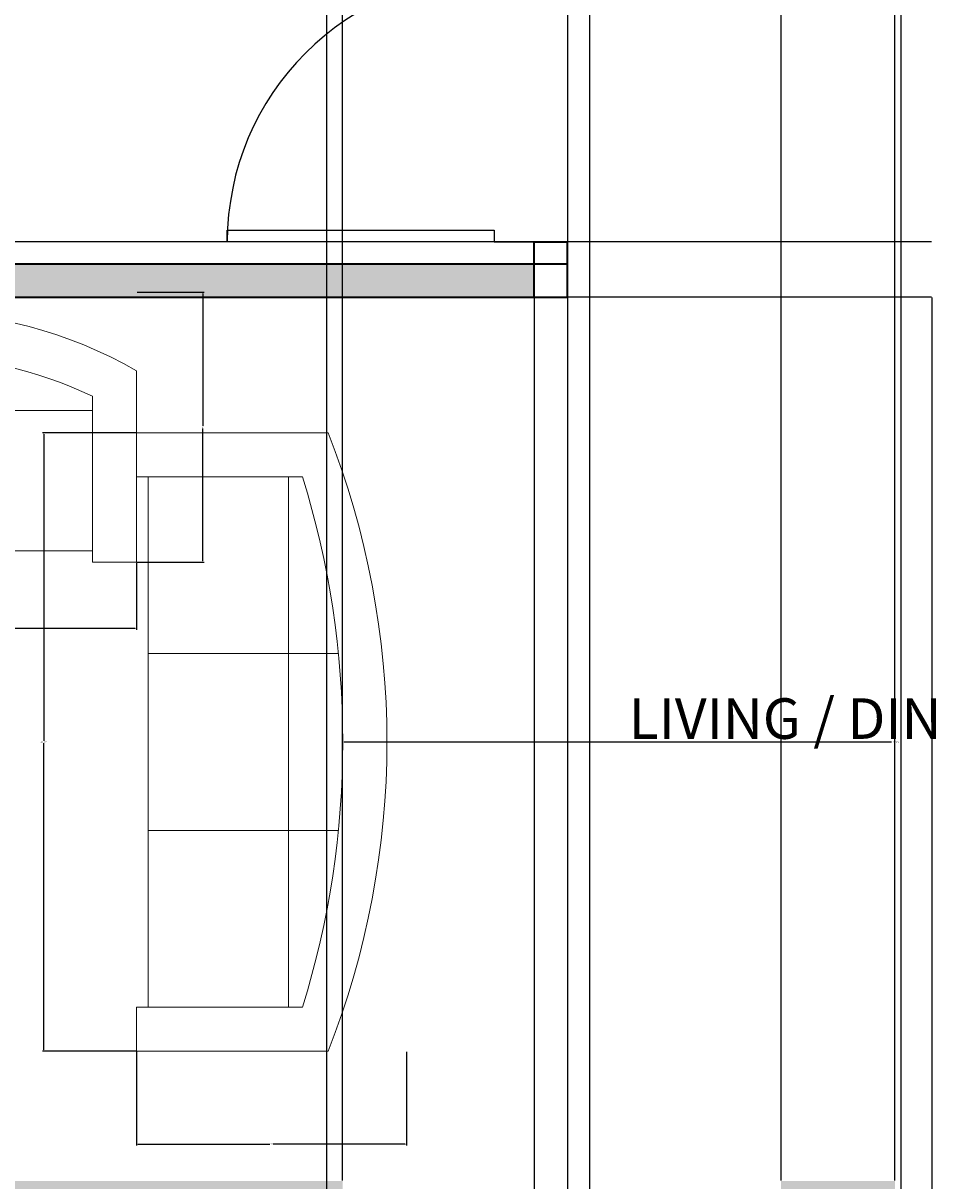
# Model space of a CAD drawing. Units: inches. Extents: x 1839 to 2285, y 722 to 1311.
# Tile 5 of 7: x 1981 to 2105, y 1018 to 1175. Entities that reach past the tile are written whole.
import ezdxf

# ---------------------------------------------------------------- set-up
doc = ezdxf.new("R2010")
doc.units = ezdxf.units.IN
for name, color, linetype, lineweight in [('A-ANNO-DIMS', 2, 'Continuous', 18), ('A-AREA-IDEN', 7, 'Continuous', 18), ('A-DOOR', 3, 'Continuous', 25), ('A-FURN', 8, 'Continuous', 18), ('A-WALL', 7, 'Continuous', 35)]:
    doc.layers.add(name, color=color, linetype=linetype, lineweight=lineweight)
doc.layers.add('A-WALL-PATT', color=18, linetype='Continuous', lineweight=13, true_color=0x000000)
doc.styles.get("Standard").update_dxf_attribs({"font": 'arial.ttf'})
doc.dimstyles.get("Standard").update_dxf_attribs({"dimtxt": 0.18, "dimasz": 0.18, "dimexe": 0.18, "dimexo": 0.0625, "dimgap": 0.09, "dimtad": 0, "dimtih": 1, "dimtoh": 1, "dimdec": 4, "dimzin": 0, "dimdsep": 46, "dimtxsty": 'Standard', "dimcen": 0.09, "dimadec": 0, "dimazin": 0, "dimtfac": 1, "dimtdec": 4, "dimtofl": 0, "dimtmove": 0, "dimatfit": 3, "dimfxl": 1, "dimtolj": 1, "dimtzin": 0, "dimarcsym": 0})

# ---------------------------------------------------------------- blocks, each defined once
blk = doc.blocks.new('*U4')
for p, q in [((0, 0), (0, -6)), ((40, 0), (40, -6))]:
    blk.add_line(p, q)
blk.add_lwpolyline([(0, 0), (0, 40), (1.75, 40), (1.75, 0)], close=True)
blk.add_arc((0, 0), 40, 0, 90)
blk = doc.blocks.new('Sofa - Roundback Loveseat 5 ft.')
for p, q in [((0, -32.44198), (0, -5.99998)), ((-24, -33.99998), (-24, -11.46958)), ((24.00004, -33.99998), (24.00004, -11.46958)), ((-23.9998, -13.38178), (23.99986, -13.38178)), ((-24, -32.44198), (24.00004, -32.44198))]:
    blk.add_line(p, q)
for points in [[(-24, -33.99998), (-30, -33.99998), (-30, -7.99998)], [(30.00004, -7.99998), (30.00004, -33.99998), (24.00004, -33.99998)]]:
    blk.add_lwpolyline(points)
for centre, radius, start, end in [((0, -60.24998), 60.24998, 60.13715, 119.8628), ((0, -61.38438), 55.38444, 64.32083, 115.6792)]:
    blk.add_arc(centre, radius, start, end)
blk = doc.blocks.new('Sofa - Roundback 7 ft.')
for p, q in [((-12.00002, -32.4421), (-12.00003, -6.5971)), ((11.99997, -32.4421), (11.99998, -6.5971)), ((-36.000027, -34), (-36.000027, -11.4696)), ((35.99998, -34), (35.99998, -11.4696)), ((-35.999844, -13.3819), (35.9998, -13.3819)), ((-36.000027, -32.4421), (35.99998, -32.4421))]:
    blk.add_line(p, q)
for points in [[(-36.000027, -34), (-42.000027, -34), (-42.000027, -8)], [(41.99998, -8), (41.99998, -34), (35.99998, -34)]]:
    blk.add_lwpolyline(points)
for centre, radius, start, end in [((0, -114.25), 114.25, 68.43141, 111.5686), ((-0.00001, -127.1968), 121.1968, 72.72033, 107.2797)]:
    blk.add_arc(centre, radius, start, end)
blk = doc.blocks.new('*D27')
at = {"layer": 'A-ANNO-DIMS', "color": 0, "lineweight": -2, "transparency": 16777216}
for p, q in [((1936.67, 1101.77), (1936.67, 1092.65)), ((1996.67, 1101.77), (1996.67, 1092.65)), ((1936.85, 1092.83), (1965.76, 1092.83)), ((1996.49, 1092.83), (1967.59, 1092.83))]:
    blk.add_line(p, q, dxfattribs=at)
at = {"layer": 'A-ANNO-DIMS', "color": 0, "transparency": 16777216}
for points in [[(1936.85, 1092.86), (1936.85, 1092.8), (1936.67, 1092.83)], [(1996.49, 1092.86), (1996.49, 1092.8), (1996.67, 1092.83)]]:
    blk.add_solid(points, dxfattribs=at)
at = {"layer": 'Defpoints', "color": 0, "transparency": 16777216}
for p in [(1936.67, 1101.83), (1996.67, 1101.83), (1996.67, 1092.83)]:
    blk.add_point(p, dxfattribs=at)
at = {"layer": 'A-ANNO-DIMS', "color": 0, "transparency": 16777216, "insert": (1966.67, 1092.83), "char_height": 0.18, "attachment_point": 5}
blk.add_mtext('\\A1;LOVESEAT 60', dxfattribs=at)
blk = doc.blocks.new('*D28')
at = {"layer": 'A-ANNO-DIMS', "color": 0, "lineweight": -2, "transparency": 16777216}
for p, q in [((1996.74, 1138.5), (2005.85, 1138.5)), ((2005.67, 1138.32), (2005.67, 1120.35)), ((2005.67, 1102.01), (2005.67, 1119.98)), ((1996.74, 1101.83), (2005.85, 1101.83))]:
    blk.add_line(p, q, dxfattribs=at)
at = {"layer": 'A-ANNO-DIMS', "color": 0, "transparency": 16777216}
for points in [[(2005.64, 1138.32), (2005.7, 1138.32), (2005.67, 1138.5)], [(2005.64, 1102.01), (2005.7, 1102.01), (2005.67, 1101.83)]]:
    blk.add_solid(points, dxfattribs=at)
at = {"layer": 'Defpoints', "color": 0, "transparency": 16777216}
for p in [(1996.67, 1138.5), (2005.67, 1138.5), (1996.67, 1101.83)]:
    blk.add_point(p, dxfattribs=at)
at = {"layer": 'A-ANNO-DIMS', "color": 0, "transparency": 16777216, "insert": (2005.67, 1120.16), "char_height": 0.18, "attachment_point": 5}
blk.add_mtext('\\A1;37', dxfattribs=at)
blk = doc.blocks.new('*D29')
at = {"layer": 'A-ANNO-DIMS', "color": 0, "lineweight": -2, "transparency": 16777216}
for p, q in [((1996.61, 1119.42), (1983.89, 1119.42)), ((1984.07, 1119.24), (1984.07, 1077.6)), ((1984.07, 1035.6), (1984.07, 1077.24)), ((1996.61, 1035.42), (1983.89, 1035.42))]:
    blk.add_line(p, q, dxfattribs=at)
at = {"layer": 'A-ANNO-DIMS', "color": 0, "transparency": 16777216}
for points in [[(1984.04, 1119.24), (1984.1, 1119.24), (1984.07, 1119.42)], [(1984.04, 1035.6), (1984.1, 1035.6), (1984.07, 1035.42)]]:
    blk.add_solid(points, dxfattribs=at)
at = {"layer": 'Defpoints', "color": 0, "transparency": 16777216}
for p in [(1996.67, 1119.42), (1984.07, 1035.42), (1996.67, 1035.42)]:
    blk.add_point(p, dxfattribs=at)
at = {"layer": 'A-ANNO-DIMS', "color": 0, "transparency": 16777216, "insert": (1984.07, 1077.42), "char_height": 0.18, "attachment_point": 5}
blk.add_mtext('\\A1;SOFA 84', dxfattribs=at)
blk = doc.blocks.new('*D30')
at = {"layer": 'A-ANNO-DIMS', "color": 0, "lineweight": -2, "transparency": 16777216}
for p, q in [((1996.67, 1035.36), (1996.67, 1022.64)), ((2033.34, 1035.36), (2033.34, 1022.64)), ((1996.85, 1022.82), (2014.79, 1022.82)), ((2033.16, 1022.82), (2015.23, 1022.82))]:
    blk.add_line(p, q, dxfattribs=at)
at = {"layer": 'A-ANNO-DIMS', "color": 0, "transparency": 16777216}
for points in [[(1996.85, 1022.85), (1996.85, 1022.79), (1996.67, 1022.82)], [(2033.16, 1022.85), (2033.16, 1022.79), (2033.34, 1022.82)]]:
    blk.add_solid(points, dxfattribs=at)
at = {"layer": 'Defpoints', "color": 0, "transparency": 16777216}
for p in [(1996.67, 1035.42), (2033.34, 1035.42), (2033.34, 1022.82)]:
    blk.add_point(p, dxfattribs=at)
at = {"layer": 'A-ANNO-DIMS', "color": 0, "transparency": 16777216, "insert": (2015.01, 1022.82), "char_height": 0.18, "attachment_point": 5}
blk.add_mtext('\\A1;37', dxfattribs=at)
blk = doc.blocks.new('*D43')
at = {"layer": 'A-ANNO-DIMS', "color": 0, "lineweight": -2, "transparency": 16777216}
for p, q in [((2050.68, 1145.27), (2050.68, 722.34)), ((1906.68, 1142.27), (1906.68, 722.34)), ((1906.86, 722.52), (1978.4, 722.52)), ((2050.5, 722.52), (1978.96, 722.52))]:
    blk.add_line(p, q, dxfattribs=at)
at = {"layer": 'A-ANNO-DIMS', "color": 0, "transparency": 16777216}
for points in [[(1906.86, 722.55), (1906.86, 722.49), (1906.68, 722.52)], [(2050.5, 722.55), (2050.5, 722.49), (2050.68, 722.52)]]:
    blk.add_solid(points, dxfattribs=at)
at = {"layer": 'Defpoints', "color": 0, "transparency": 16777216}
for p in [(2050.68, 1145.33), (1906.68, 1142.33), (2050.68, 722.52)]:
    blk.add_point(p, dxfattribs=at)
at = {"layer": 'A-ANNO-DIMS', "color": 0, "transparency": 16777216, "insert": (1978.68, 722.52), "char_height": 0.18, "attachment_point": 5}
blk.add_mtext('\\A1;144', dxfattribs=at)
blk = doc.blocks.new('*D44')
at = {"layer": 'A-ANNO-DIMS', "color": 0, "lineweight": -2, "transparency": 16777216}
for p, q in [((2055.18, 1137.77), (2055.18, 722.34)), ((2104.68, 1137.77), (2104.68, 722.34)), ((2055.36, 722.52), (2079.6, 722.52)), ((2104.5, 722.52), (2080.26, 722.52))]:
    blk.add_line(p, q, dxfattribs=at)
at = {"layer": 'A-ANNO-DIMS', "color": 0, "transparency": 16777216}
for points in [[(2055.36, 722.55), (2055.36, 722.49), (2055.18, 722.52)], [(2104.5, 722.55), (2104.5, 722.49), (2104.68, 722.52)]]:
    blk.add_solid(points, dxfattribs=at)
at = {"layer": 'Defpoints', "color": 0, "transparency": 16777216}
for p in [(2055.18, 1137.83), (2104.68, 1137.83), (2104.68, 722.52)]:
    blk.add_point(p, dxfattribs=at)
at = {"layer": 'A-ANNO-DIMS', "color": 0, "transparency": 16777216, "insert": (2079.93, 722.52), "char_height": 0.18, "attachment_point": 5}
blk.add_mtext('\\A1;49.5', dxfattribs=at)
blk = doc.blocks.new('*D53')
at = {"layer": 'A-ANNO-DIMS', "color": 0, "lineweight": -2, "transparency": 16777216}
for p, q in [((2099.66, 1017.89), (2099.66, 1310.76)), ((2099.84, 1310.58), (2129.54, 1310.58)), ((2160, 1310.58), (2130.3, 1310.58)), ((2160.18, 1017.89), (2160.18, 1310.76))]:
    blk.add_line(p, q, dxfattribs=at)
at = {"layer": 'A-ANNO-DIMS', "color": 0, "transparency": 16777216}
for points in [[(2099.84, 1310.61), (2099.84, 1310.55), (2099.66, 1310.58)], [(2160, 1310.61), (2160, 1310.55), (2160.18, 1310.58)]]:
    blk.add_solid(points, dxfattribs=at)
at = {"layer": 'Defpoints', "color": 0, "transparency": 16777216}
for p in [(2160.18, 1310.58), (2099.66, 1017.83), (2160.18, 1017.83)]:
    blk.add_point(p, dxfattribs=at)
at = {"layer": 'A-ANNO-DIMS', "color": 0, "transparency": 16777216, "insert": (2129.92, 1310.58), "char_height": 0.18, "attachment_point": 5}
blk.add_mtext('\\A1;60.51', dxfattribs=at)
blk = doc.blocks.new('*D55')
at = {"layer": 'A-ANNO-DIMS', "color": 0, "lineweight": -2, "transparency": 16777216}
for p, q in [((2022.5, 812.39), (2022.5, 1310.76)), ((2022.68, 1310.58), (2061.29, 1310.58)), ((2100.32, 1310.58), (2061.72, 1310.58)), ((2100.5, 812.39), (2100.5, 1310.76))]:
    blk.add_line(p, q, dxfattribs=at)
at = {"layer": 'A-ANNO-DIMS', "color": 0, "transparency": 16777216}
for points in [[(2022.68, 1310.61), (2022.68, 1310.55), (2022.5, 1310.58)], [(2100.32, 1310.61), (2100.32, 1310.55), (2100.5, 1310.58)]]:
    blk.add_solid(points, dxfattribs=at)
at = {"layer": 'Defpoints', "color": 0, "transparency": 16777216}
for p in [(2100.5, 1310.58), (2022.5, 812.33), (2100.5, 812.33)]:
    blk.add_point(p, dxfattribs=at)
at = {"layer": 'A-ANNO-DIMS', "color": 0, "transparency": 16777216, "insert": (2061.5, 1310.58), "char_height": 0.18, "attachment_point": 5}
blk.add_mtext('\\A1;78', dxfattribs=at)
blk = doc.blocks.new('*D59')
at = {"layer": 'A-ANNO-DIMS', "color": 0, "lineweight": -2, "transparency": 16777216}
for p, q in [((2024.66, 1017.89), (2024.66, 1310.76)), ((2024.84, 1310.58), (2054.04, 1310.58)), ((2084.02, 1310.58), (2054.82, 1310.58)), ((2084.2, 1017.89), (2084.2, 1310.76))]:
    blk.add_line(p, q, dxfattribs=at)
at = {"layer": 'A-ANNO-DIMS', "color": 0, "transparency": 16777216}
for points in [[(2024.84, 1310.61), (2024.84, 1310.55), (2024.66, 1310.58)], [(2084.02, 1310.61), (2084.02, 1310.55), (2084.2, 1310.58)]]:
    blk.add_solid(points, dxfattribs=at)
at = {"layer": 'Defpoints', "color": 0, "transparency": 16777216}
for p in [(2084.2, 1310.58), (2024.66, 1017.83), (2084.2, 1017.83)]:
    blk.add_point(p, dxfattribs=at)
at = {"layer": 'A-ANNO-DIMS', "color": 0, "transparency": 16777216, "insert": (2054.43, 1310.58), "char_height": 0.18, "attachment_point": 5}
blk.add_mtext('\\A1;59.53', dxfattribs=at)
blk = doc.blocks.new('*D66')
at = {"layer": 'A-ANNO-DIMS', "color": 0, "lineweight": -2, "transparency": 16777216}
for p, q in [((1975.68, 1017.89), (1975.68, 1310.76)), ((1975.86, 1310.58), (1999.77, 1310.58)), ((2024.48, 1310.58), (2000.57, 1310.58)), ((2024.66, 1017.89), (2024.66, 1310.76))]:
    blk.add_line(p, q, dxfattribs=at)
at = {"layer": 'A-ANNO-DIMS', "color": 0, "transparency": 16777216}
for points in [[(1975.86, 1310.61), (1975.86, 1310.55), (1975.68, 1310.58)], [(2024.48, 1310.61), (2024.48, 1310.55), (2024.66, 1310.58)]]:
    blk.add_solid(points, dxfattribs=at)
at = {"layer": 'Defpoints', "color": 0, "transparency": 16777216}
for p in [(2024.66, 1310.58), (1975.68, 1017.83), (2024.66, 1017.83)]:
    blk.add_point(p, dxfattribs=at)
at = {"layer": 'A-ANNO-DIMS', "color": 0, "transparency": 16777216, "insert": (2000.17, 1310.58), "char_height": 0.18, "attachment_point": 5}
blk.add_mtext('\\A1;48.99', dxfattribs=at)
blk = doc.blocks.new('*D70')
at = {"layer": 'A-ANNO-DIMS', "color": 0, "lineweight": -2, "transparency": 16777216}
for p, q in [((2104.61, 1181.33), (1870.25, 1181.33)), ((1870.43, 1181.15), (1870.43, 1163.51)), ((1870.43, 1145.51), (1870.43, 1163.15)), ((2104.61, 1145.33), (1870.25, 1145.33))]:
    blk.add_line(p, q, dxfattribs=at)
at = {"layer": 'A-ANNO-DIMS', "color": 0, "transparency": 16777216}
for points in [[(1870.4, 1181.15), (1870.46, 1181.15), (1870.43, 1181.33)], [(1870.4, 1145.51), (1870.46, 1145.51), (1870.43, 1145.33)]]:
    blk.add_solid(points, dxfattribs=at)
at = {"layer": 'Defpoints', "color": 0, "transparency": 16777216}
for p in [(1870.43, 1181.33), (2104.68, 1181.33), (2104.68, 1145.33)]:
    blk.add_point(p, dxfattribs=at)
at = {"layer": 'A-ANNO-DIMS', "color": 0, "transparency": 16777216, "insert": (1870.43, 1163.33), "char_height": 0.18, "attachment_point": 5}
blk.add_mtext('\\A1;36', dxfattribs=at)
blk = doc.blocks.new('*D83')
at = {"layer": 'A-ANNO-DIMS', "color": 0, "lineweight": -2, "transparency": 16777216}
for p, q in [((2104.61, 1145.33), (1870.25, 1145.33)), ((1870.43, 1145.15), (1870.43, 1141.76)), ((1870.43, 1138.01), (1870.43, 1141.4)), ((2104.61, 1137.83), (1870.25, 1137.83))]:
    blk.add_line(p, q, dxfattribs=at)
at = {"layer": 'A-ANNO-DIMS', "color": 0, "transparency": 16777216}
for points in [[(1870.4, 1145.15), (1870.46, 1145.15), (1870.43, 1145.33)], [(1870.4, 1138.01), (1870.46, 1138.01), (1870.43, 1137.83)]]:
    blk.add_solid(points, dxfattribs=at)
at = {"layer": 'Defpoints', "color": 0, "transparency": 16777216}
for p in [(1870.43, 1145.33), (2104.68, 1145.33), (2104.68, 1137.83)]:
    blk.add_point(p, dxfattribs=at)
at = {"layer": 'A-ANNO-DIMS', "color": 0, "transparency": 16777216, "insert": (1870.43, 1141.58), "char_height": 0.18, "attachment_point": 5}
blk.add_mtext('\\A1;7.5', dxfattribs=at)
blk = doc.blocks.new('*D84')
at = {"layer": 'A-ANNO-DIMS', "color": 0, "lineweight": -2, "transparency": 16777216}
for p, q in [((2055.18, 1218.77), (2055.18, 722.34)), ((2058.18, 1218.77), (2058.18, 722.34)), ((2055.36, 722.52), (2056.53, 722.52)), ((2058, 722.52), (2056.83, 722.52))]:
    blk.add_line(p, q, dxfattribs=at)
at = {"layer": 'A-ANNO-DIMS', "color": 0, "transparency": 16777216}
for points in [[(2055.36, 722.55), (2055.36, 722.49), (2055.18, 722.52)], [(2058, 722.55), (2058, 722.49), (2058.18, 722.52)]]:
    blk.add_solid(points, dxfattribs=at)
at = {"layer": 'Defpoints', "color": 0, "transparency": 16777216}
for p in [(2055.18, 1218.83), (2058.18, 1218.83), (2058.18, 722.52)]:
    blk.add_point(p, dxfattribs=at)
at = {"layer": 'A-ANNO-DIMS', "color": 0, "transparency": 16777216, "insert": (2056.68, 722.52), "char_height": 0.18, "attachment_point": 5}
blk.add_mtext('\\A1;3', dxfattribs=at)
blk = doc.blocks.new('*D86')
at = {"layer": 'A-ANNO-DIMS', "color": 0, "lineweight": -2, "transparency": 16777216}
for p, q in [((1903.39, 1077.42), (1903.57, 1077.42)), ((1903.48, 1077.33), (1903.48, 1077.51)), ((2097.39, 1077.42), (2024.85, 1077.42))]:
    blk.add_line(p, q, dxfattribs=at)
at = {"layer": 'A-ANNO-DIMS', "color": 0, "transparency": 16777216}
blk.add_solid([(2024.85, 1077.45), (2024.85, 1077.39), (2024.67, 1077.42)], dxfattribs=at)
at = {"layer": 'Defpoints', "color": 0, "transparency": 16777216}
for p in [(1903.48, 1077.42), (2024.67, 1077.42)]:
    blk.add_point(p, dxfattribs=at)
at = {"layer": 'A-ANNO-DIMS', "color": 0, "transparency": 16777216, "insert": (2097.87, 1077.42), "char_height": 0.18, "attachment_point": 5}
blk.add_mtext('\\A1;R121.2', dxfattribs=at)
blk = doc.blocks.new('*D87')
at = {"layer": 'A-ANNO-DIMS', "color": 0, "lineweight": -2, "transparency": 16777216}
for p, q in [((1916.33, 1077.42), (1916.51, 1077.42)), ((1916.42, 1077.33), (1916.42, 1077.51)), ((2099.22, 1077.42), (2030.85, 1077.42))]:
    blk.add_line(p, q, dxfattribs=at)
at = {"layer": 'A-ANNO-DIMS', "color": 0, "transparency": 16777216}
blk.add_solid([(2030.85, 1077.45), (2030.85, 1077.39), (2030.67, 1077.42)], dxfattribs=at)
at = {"layer": 'Defpoints', "color": 0, "transparency": 16777216}
for p in [(1916.42, 1077.42), (2030.67, 1077.42)]:
    blk.add_point(p, dxfattribs=at)
at = {"layer": 'A-ANNO-DIMS', "color": 0, "transparency": 16777216, "insert": (2099.77, 1077.42), "char_height": 0.18, "attachment_point": 5}
blk.add_mtext('\\A1;R114.25', dxfattribs=at)

msp = doc.modelspace()

# ---------------------------------------------------------------- hatches: boundary and pattern name
at = {"layer": 'A-WALL-PATT'}
h = msp.add_hatch(color=256, dxfattribs=at)
h.dxf.hatch_style = 1
h.paths.add_polyline_path([(1906.6771, 1274.3314), (1942.6771, 1274.3314), (1942.6771, 1283.3314), (1897.6771, 1283.3314), (1897.6771, 968.2107), (1906.6771, 968.2107), (1906.6771, 1013.3314), (1939.6771, 1013.3314), (1939.6771, 1017.8314), (1906.6771, 1017.8314), (1906.6771, 1137.8314), (2050.6771, 1137.8314), (2050.6771, 1142.3314), (1906.6771, 1142.3314)])
h.paths.add_polyline_path([(2064.0508, 1283.3314), (1978.6771, 1283.3314), (1978.6771, 1274.3314), (2050.6771, 1274.3314), (2050.6771, 1184.3314), (2055.1771, 1184.3314), (2055.1771, 1214.3314), (2058.1771, 1214.3314), (2058.1771, 1218.8314), (2055.1771, 1218.8314), (2055.1771, 1274.3314), (2064.0508, 1274.3314)])
h.paths.add_polyline_path([(2182.6416, 1283.3314), (2088.0508, 1283.3314), (2088.0508, 1274.3314), (2104.6771, 1274.3314), (2104.6771, 1218.8314), (2094.1771, 1218.8314), (2094.1771, 1214.3314), (2104.6771, 1214.3314), (2104.6771, 1184.3314), (2109.1771, 1184.3314), (2109.1771, 1274.3314), (2182.6416, 1274.3314)])
h.paths.add_polyline_path([(2257.6771, 1283.3314), (2218.6416, 1283.3314), (2218.6416, 1274.3314), (2248.6771, 1274.3314), (2248.6771, 1142.3314), (2186.4004, 1142.3314), (2109.1771, 1142.3314), (2109.1771, 1137.8314), (2248.6771, 1137.8314), (2248.6771, 1094.9086), (2257.6771, 1094.9086)])
h.paths.add_polyline_path([(2257.6771, 1058.9086), (2248.6771, 1058.9086), (2248.6771, 1017.8314), (2160.1771, 1017.8314), (2160.1771, 939.8314), (2164.6771, 939.8314), (2164.6771, 1013.3314), (2248.6771, 1013.3314), (2248.6771, 977.3314), (2248.6771, 950.4862), (2257.6771, 950.4862)])
h.paths.add_polyline_path([(2257.6771, 893.3314), (2248.6771, 893.3314), (2248.6771, 850.1143), (2190.4862, 850.1143), (2190.4862, 845.6143), (2248.6771, 845.6143), (2248.6771, 812.3314), (2100.5038, 812.3314), (2100.5038, 803.3314), (2257.6771, 803.3314)])
h.paths.add_polyline_path([(2257.6771, 926.4862), (2248.6771, 926.4862), (2248.6771, 897.8314), (2141.6642, 897.8314), (2141.6642, 893.3314), (2145.5038, 893.3314), (2145.5038, 812.3314), (2147.5038, 812.3314), (2147.5038, 845.6143), (2153.9854, 845.6143), (2153.9854, 850.1143), (2147.5038, 850.1143), (2147.5038, 893.3314), (2248.6771, 893.3314), (2257.6771, 893.3314)])
h.paths.add_polyline_path([(1906.6771, 893.3314), (1897.6771, 893.3314), (1897.6771, 803.3314), (2022.5038, 803.3314), (2022.5038, 812.3314), (1906.6771, 812.3314)])
h.paths.add_polyline_path([(2031.4676, 897.8314), (1981.6771, 897.8314), (1981.6771, 1013.3314), (2024.6642, 1013.3314), (2024.6642, 1017.8314), (1975.6771, 1017.8314), (1975.6771, 1013.3314), (1978.6771, 1013.3314), (1978.6771, 897.8314), (1906.6771, 897.8314), (1906.6771, 932.2107), (1897.6771, 932.2107), (1897.6771, 893.3314), (1906.6771, 893.3314), (2031.4676, 893.3314)])
h.paths.add_polyline_path([(2099.6642, 1017.8314), (2096.6642, 1017.8314), (2084.1956, 1017.8314), (2084.1956, 1013.3314), (2096.6642, 1013.3314), (2096.6642, 897.8314), (2085.6129, 897.8314), (2085.6129, 893.3314), (2102.6642, 893.3314), (2102.6642, 897.8314), (2099.6642, 897.8314)])

# ---------------------------------------------------------------- linework, layer by layer
at = {"layer": 'A-WALL'}
for p, q in [((2050.6771, 1137.8314), (2050.6771, 1145.3314)), ((2050.6771, 1145.3314), (2055.1771, 1145.3314)), ((2055.1771, 1137.8314), (2055.1771, 1145.3314)), ((1906.6771, 1142.3314), (2055.1771, 1142.3314)), ((1906.6771, 1137.8314), (2055.1771, 1137.8314))]:
    msp.add_line(p, q, dxfattribs=at)

# ---------------------------------------------------------------- block references
at = {"layer": 'A-DOOR', "xscale": 0.9062393225401889, "yscale": 0.9062393225401889, "zscale": 0.9062393225401889, "rotation": 90}
msp.add_blockref('*U4', (2045.2397, 1145.3314), dxfattribs=at)
at = {"layer": 'A-FURN'}
msp.add_blockref('Sofa - Roundback Loveseat 5 ft.', (1966.6741, 1135.8314), dxfattribs=at)
at = {"layer": 'A-FURN', "rotation": 270}
msp.add_blockref('Sofa - Roundback 7 ft.', (2030.6742, 1077.4214), dxfattribs=at)

# ---------------------------------------------------------------- texts
at = {"layer": 'A-AREA-IDEN'}
msp.add_text('LIVING / DINING ', height=5.503795, dxfattribs=at).set_placement((2063.4967, 1077.8469))

# ---------------------------------------------------------------- dimensions: what is measured, and where the dimension line sits
at = {"layer": 'A-ANNO-DIMS'}
for base, p1, p2, override, picture, middle in [((2024.6642, 1310.5814), (1975.6771, 1017.8314), (2024.6642, 1017.8314), {"dimdec": 2, "dimlfac": 1, "dimrnd": 0, "dimzin": 0, "dimdsep": 46, "dimlunit": 2}, '*D66', (2000.1706, 1310.5814)), ((2100.5038, 1310.5814), (2022.5038, 812.3314), (2100.5038, 812.3314), {"dimdec": 0, "dimlfac": 1, "dimrnd": 0, "dimzin": 0, "dimdsep": 46, "dimlunit": 2}, '*D55', (2061.5038, 1310.5814)), ((2084.1956, 1310.5814), (2024.6642, 1017.8314), (2084.1956, 1017.8314), {"dimdec": 2, "dimlfac": 1, "dimrnd": 0, "dimzin": 0, "dimdsep": 46, "dimlunit": 2}, '*D59', (2054.4299, 1310.5814)), ((2160.1771, 1310.5814), (2099.6642, 1017.8314), (2160.1771, 1017.8314), {"dimdec": 2, "dimlfac": 1, "dimrnd": 0, "dimzin": 0, "dimdsep": 46, "dimlunit": 2}, '*D53', (2129.9206, 1310.5814)), ((2058.1771, 722.516), (2055.1771, 1218.8314), (2058.1771, 1218.8314), {"dimdec": 0, "dimlfac": 1, "dimrnd": 0, "dimzin": 0, "dimdsep": 46, "dimlunit": 2}, '*D84', (2056.6771, 722.516)), ((2050.6771, 722.516), (1906.6771, 1142.3314), (2050.6771, 1145.3314), {"dimdec": 0, "dimlfac": 1, "dimrnd": 0, "dimzin": 0, "dimdsep": 46, "dimlunit": 2}, '*D43', (1978.6771, 722.516)), ((2104.6771, 722.516), (2055.1771, 1137.8314), (2104.6771, 1137.8314), {"dimdec": 1, "dimlfac": 1, "dimrnd": 0, "dimzin": 0, "dimdsep": 46, "dimlunit": 2}, '*D44', (2079.9271, 722.516)), ((2033.3408, 1022.8214), (1996.6742, 1035.4214), (2033.3408, 1035.4214), {"dimdec": 0, "dimlfac": 1, "dimrnd": 0, "dimzin": 0, "dimdsep": 46, "dimlunit": 2}, '*D30', (2015.0075, 1022.8214))]:
    dim = msp.add_linear_dim(base=base, p1=p1, p2=p2, dimstyle='Standard', override=override, dxfattribs=at)
    dim.commit()
    dim.dimension.update_dxf_attribs({"geometry": picture, "text_midpoint": middle})
for base, p1, p2, override, picture, middle in [((1870.4271, 1181.3314), (2104.6771, 1145.3314), (2104.6771, 1181.3314), {"dimdec": 0, "dimlfac": 1, "dimrnd": 0, "dimzin": 0, "dimdsep": 46, "dimlunit": 2}, '*D70', (1870.4271, 1163.3314)), ((1870.4271, 1145.3314), (2104.6771, 1137.8314), (2104.6771, 1145.3314), {"dimdec": 1, "dimlfac": 1, "dimrnd": 0, "dimzin": 0, "dimdsep": 46, "dimlunit": 2}, '*D83', (1870.4271, 1141.5814)), ((2005.6742, 1138.4981), (1996.6742, 1101.8314), (1996.6742, 1138.4981), {"dimdec": 0, "dimlfac": 1, "dimrnd": 0, "dimzin": 0, "dimdsep": 46, "dimlunit": 2}, '*D28', (2005.6742, 1120.1648))]:
    dim = msp.add_linear_dim(base=base, p1=p1, p2=p2, angle=90, dimstyle='Standard', override=override, dxfattribs=at)
    dim.commit()
    dim.dimension.update_dxf_attribs({"geometry": picture, "text_midpoint": middle})
dim = msp.add_linear_dim(base=(1984.0742, 1035.4214), p1=(1996.6742, 1119.4214), p2=(1996.6742, 1035.4214), angle=270, text='SOFA <>', dimstyle='Standard', override={"dimdec": 0, "dimlfac": 1, "dimrnd": 0, "dimzin": 0, "dimdsep": 46, "dimlunit": 2}, dxfattribs=at)
dim.commit()
dim.dimension.update_dxf_attribs({"geometry": '*D29', "text_midpoint": (1984.0742, 1077.4214)})
dim = msp.add_linear_dim(base=(1996.6742, 1092.8314), p1=(1936.6741, 1101.8314), p2=(1996.6742, 1101.8314), text='LOVESEAT <>', dimstyle='Standard', override={"dimdec": 0, "dimlfac": 1, "dimrnd": 0, "dimzin": 0, "dimdsep": 46, "dimlunit": 2}, dxfattribs=at)
dim.commit()
dim.dimension.update_dxf_attribs({"geometry": '*D27', "text_midpoint": (1966.6741, 1092.8314)})
for center, mpoint, override, picture, middle in [((1903.4774, 1077.4214), (2024.6742, 1077.421), {"dimdec": 1, "dimlfac": 1, "dimrnd": 0, "dimzin": 0, "dimdsep": 46, "dimlunit": 2}, '*D86', (2097.3922, 1077.4208)), ((1916.4242, 1077.4214), (2030.6742, 1077.421), {"dimdec": 2, "dimlfac": 1, "dimrnd": 0, "dimzin": 0, "dimdsep": 46, "dimlunit": 2}, '*D87', (2099.2242, 1077.4208))]:
    dim = msp.add_radius_dim(center=center, mpoint=mpoint, dimstyle='Standard', override=override, dxfattribs=at)
    dim.commit()
    dim.dimension.update_dxf_attribs({"geometry": picture, "text_midpoint": middle, "dimtype": 164})

doc.saveas('drawing.dxf')
